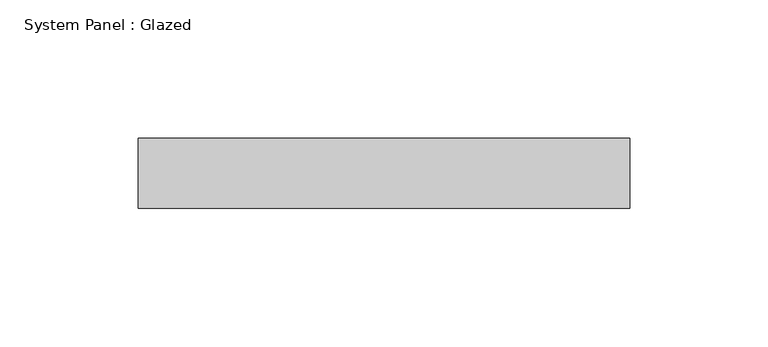
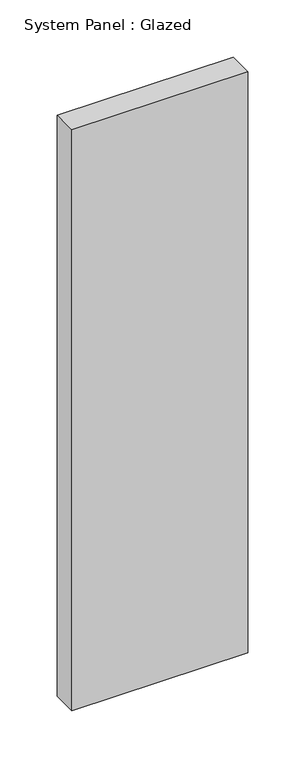
"""IFC4 building model written with IfcOpenShell, lengths in millimetres: plate geometry, System Panel : Glazed."""

from ifc_helpers import new_model, si_unit, origin, origin_with_axes, place, context, project, spatial, polyline, outline, extrude, source, transform, mapped, element, save


def system_panel_glazed_879596d7(model_context):
    return source(origin(), model_context, "Body", "SweptSolid", [
        extrude(outline(polyline([(88.9, 19.05), (-88.9, 19.05), (-88.9, 44.45), (88.9, 44.45), (88.9, 19.05)])), origin_with_axes(), (0.0, 0.0, 1.0), 620.2625925),
    ])


if __name__ == "__main__":
    model = new_model("IFC4")
    model_context = context("Model", 3, world=origin())
    ifc_project = project(units=[si_unit("LENGTHUNIT", "METRE", prefix="MILLI")], contexts=[model_context])
    site = spatial("IfcSite", under=ifc_project)
    building = spatial("IfcBuilding", under=site)
    placement = place(None, origin())
    system_panel_glazed_shape = system_panel_glazed_879596d7(model_context)
    element("IfcPlate", 1, ObjectType="System Panel : Glazed", at=placement, inside=building, context=model_context, shape_type="MappedRepresentation", body=[
        mapped(system_panel_glazed_shape, transform((0.0, 0.0, 0.0), x_axis=(1.0, 0.0, 0.0), y_axis=(0.0, 1.0, 0.0), z_axis=(0.0, 0.0, 1.0))),
    ])
    save(model, "model.ifc")

# Revit data of these elements
# Type "System Panel : Glazed"
#   Construction Type Id = "GSP4R"
#   Analytic Construction = "1/8 in Pilkington single glazing"
#   Visual Light Transmittance = 0.9
#   Solar Heat Gain Coefficient = 0.86
#   Heat Transfer Coefficient (U) = 1.18115 BTU/(h·ft²·°F)
#   Define Thermal Properties by = 1
# Element 1 (IfcPlate, "System Panel : Glazed")
#   Materials on its faces: "Glass"
# Materials
#   "Glass": class "Glass", colour RGB 0 128 192, transparency 0.75, Description = "Soda Lime Glass", Cost = 0
